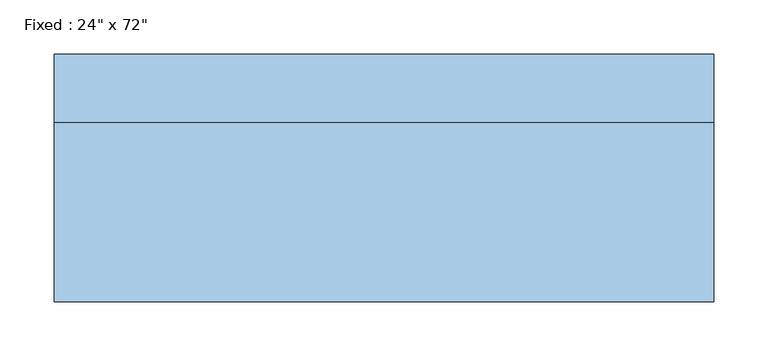
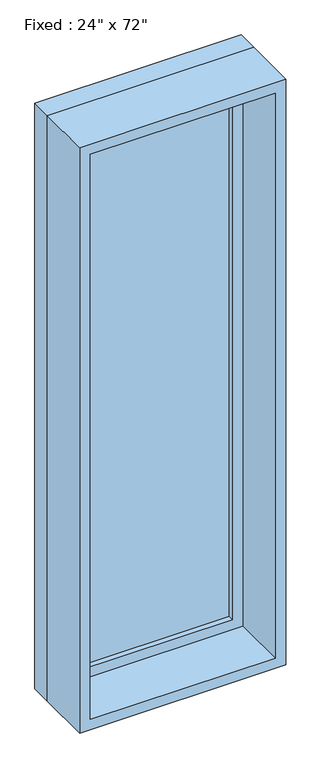
"""IFC4 building model written with IfcOpenShell, lengths in millimetres: window geometry."""

from ifc_helpers import new_model, si_unit, frame, origin, place, context, project, spatial, polyline, outline, extrude, source, transform, mapped, element, save


def window_fc882ab3(model_context):
    return source(origin(), model_context, "Body", "SweptSolid", [
        extrude(outline(polyline([(203.2, 66.675), (-279.4, 66.675), (-279.4, 79.375), (203.2, 79.375), (203.2, 66.675)])), frame((0.0, 0.0, 368.3), z_axis=(0.0, 0.0, 1.0), x_axis=(1.0, 0.0, 0.0)), (0.0, 0.0, 1.0), 1701.8),
        extrude(outline(polyline([(2114.55, -323.85), (323.85, -323.85), (323.85, 247.65), (2114.55, 247.65), (2114.55, -323.85)]), holes=[polyline([(2070.1, -279.4), (2070.1, 203.2), (368.3, 203.2), (368.3, -279.4), (2070.1, -279.4)])]), frame((0.0, 50.8, 0.0), z_axis=(0.0, 1.0, 0.0), x_axis=(0.0, 0.0, 1.0)), (0.0, 0.0, 1.0), 44.45),
        extrude(outline(polyline([(2133.6, -342.9), (304.8, -342.9), (304.8, 266.7), (2133.6, 266.7), (2133.6, -342.9)]), holes=[polyline([(2101.85, -311.15), (2101.85, 234.95), (336.55, 234.95), (336.55, -311.15), (2101.85, -311.15)])]), frame((0.0, -114.3, 0.0), z_axis=(0.0, 1.0, 0.0), x_axis=(0.0, 0.0, 1.0)), (0.0, 0.0, 1.0), 165.1),
        extrude(outline(polyline([(2133.6, 266.7), (2133.6, -342.9), (304.8, -342.9), (304.8, 266.7), (2133.6, 266.7)]), holes=[polyline([(2114.55, 247.65), (323.85, 247.65), (323.85, -323.85), (2114.55, -323.85), (2114.55, 247.65)])]), frame((0.0, 50.8, 0.0), z_axis=(0.0, 1.0, 0.0), x_axis=(0.0, 0.0, 1.0)), (0.0, 0.0, 1.0), 63.5),
    ])


if __name__ == "__main__":
    model = new_model("IFC4")
    model_context = context("Model", 3, world=origin())
    ifc_project = project(units=[si_unit("LENGTHUNIT", "METRE", prefix="MILLI")], contexts=[model_context])
    site = spatial("IfcSite", under=ifc_project)
    building = spatial("IfcBuilding", under=site)
    placement = place(None, origin())
    window_shape = window_fc882ab3(model_context)
    element("IfcWindow", 1, ObjectType="Fixed : 24\" x 72\"", at=placement, inside=building, context=model_context, shape_type="MappedRepresentation", body=[
        mapped(window_shape, transform((0.0, 0.0, 0.0), x_axis=(1.0, 0.0, 0.0), y_axis=(0.0, 1.0, 0.0), z_axis=(0.0, 0.0, 1.0))),
    ])
    save(model, "model.ifc")

# Revit data of these elements
# Type "Fixed : 24\" x 72\""
#   Type Mark = "7"
#   Assembly Code = "B2020100"
#   Height = 6' - 0"
#   Default Sill Height = 1' - 0"
#   Width = 2' - 0"
#   Window Inset = 0' - 0 3/4"
#   Glass Pane Material = Glass
#   Sash Material = Sash
#   Wall Closure = (empty or 0)
# Element 1 (IfcWindow, "Fixed : 24\" x 72\"")
#   Materials on its faces: "Sash", "Glass"
# Materials
#   "Glass": class "Glass", colour RGB 218 227 224, transparency 0.85, Description = "Soda Lime Glass", Cost = 0
#   "Sash": class "Wood", colour RGB 136 99 55, transparency 0
